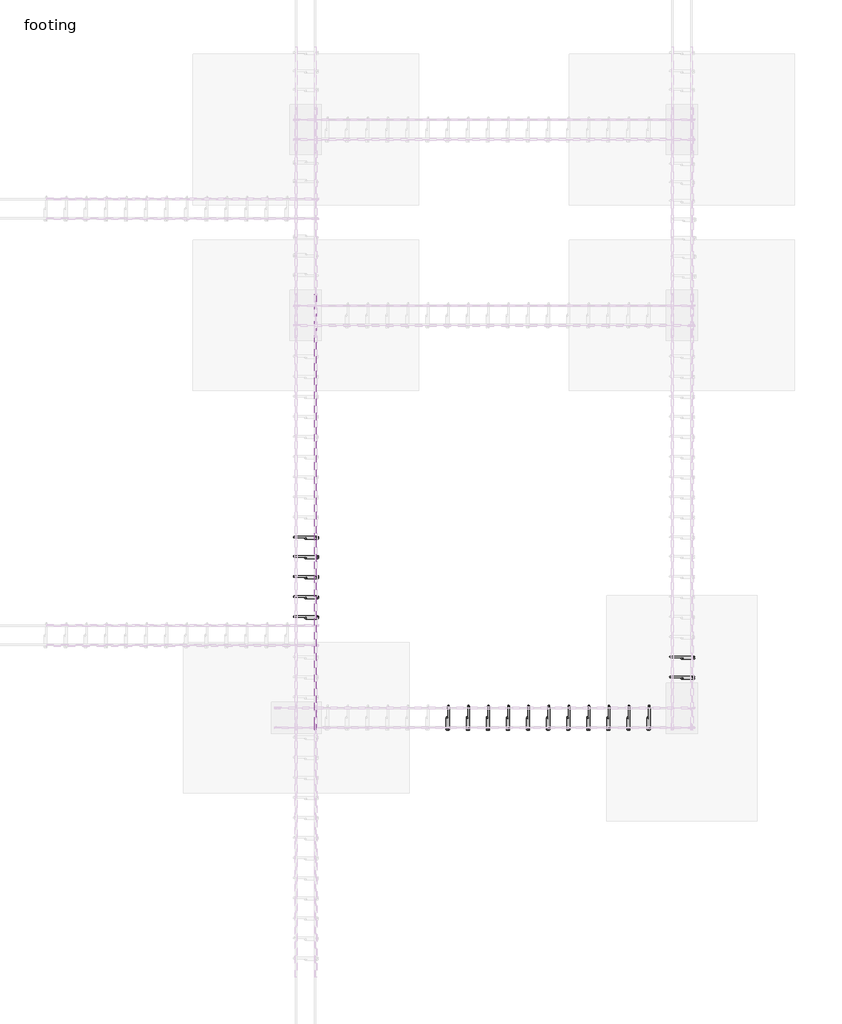
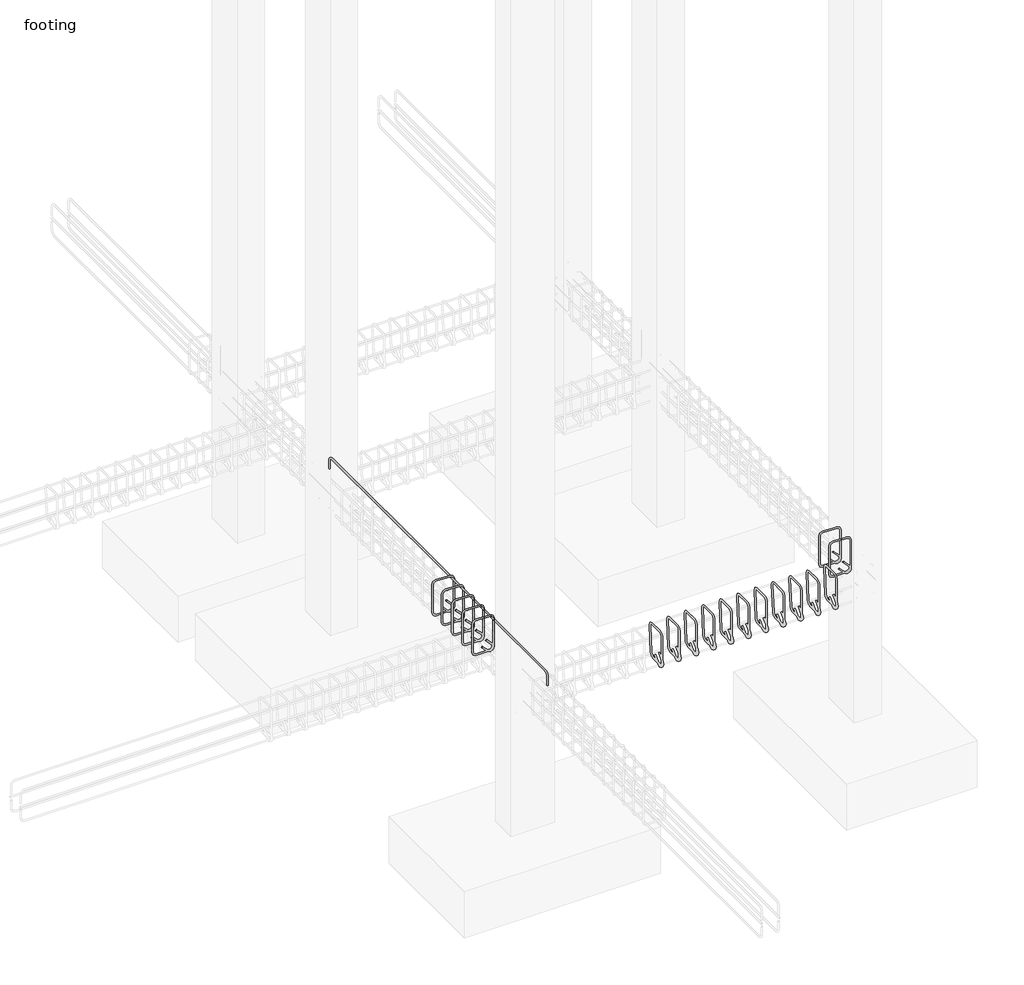
# One storey, part 11 of 21: 19 reinforcing bars.
"""IFC4 building model written with IfcOpenShell, lengths in millimetres."""

from ifc_helpers import new_model, si_unit, point, frame, origin, place, context, project, spatial, polyline, circle_curve, trimmed, segment, composite_curve, element, save
from ifc_brep_helpers import swept_disk

model = new_model("IFC4")

# Units and contexts
model_context = context("Model", 3, world=origin())
ifc_project = project(units=[si_unit("LENGTHUNIT", "METRE", prefix="MILLI")], contexts=[model_context])

# Site, building, storey
site = spatial("IfcSite", under=ifc_project)
building = spatial("IfcBuilding", under=site)
storey = spatial("IfcBuildingStorey", under=building, Name="footing", Elevation=-1524.0)

# Reinforcing bars
placement = place(None, origin())
element("IfcReinforcingBar", 1, at=placement, inside=storey, context=model_context, shape_type="SolidModel", body=[
    swept_disk(composite_curve([segment(polyline([(-6723.5883428, 3451.1387132, -310.8825168), (-6723.5883428, 3396.2737147, -365.7475153)]), True, "CONTINUOUS"), segment(trimmed(circle_curve(frame((-6723.5883428, 3373.8230744, -343.296875), z_axis=(-1.0, 0.0, 0.0), x_axis=(0.0, 22.450640299999577, -22.450640299999975)), 31.75), [point((-6723.5883428, 3396.2737147, -365.7475153))], [point((-6723.5883428, 3342.0730744, -343.296875))], True, "CARTESIAN"), True, "CONTINUOUS"), segment(polyline([(-6723.5883428, 3342.0730744, -343.296875), (-6723.5883428, 3342.0730744, -63.103125)]), True, "CONTINUOUS"), segment(trimmed(circle_curve(frame((-6723.5883428, 3373.8230744, -63.103125), z_axis=(-1.0, 0.0, 0.0), x_axis=(0.0, -31.75, 0.0)), 31.75), [point((-6723.5883428, 3342.0730744, -63.103125))], [point((-6723.5883428, 3373.8230744, -31.353125))], True, "CARTESIAN"), True, "CONTINUOUS"), segment(polyline([(-6723.5883428, 3373.8230744, -31.353125), (-6723.5883428, 3501.6168244, -31.353125)]), True, "CONTINUOUS"), segment(trimmed(circle_curve(frame((-6722.4159328, 3501.6168244, -63.0814712), z_axis=(-0.9993179916193466, 0.0, -0.03692629992126919), x_axis=(-1.1724100000001272, 0.0, 31.728346200000004)), 31.75), [point((-6723.5883428, 3501.6168244, -31.353125))], [point((-6722.4159328, 3533.3668244, -63.0814712))], True, "CARTESIAN"), True, "CONTINUOUS"), segment(polyline([(-6722.4159328, 3533.3668244, -63.0814712), (-6712.0607528, 3533.3668244, -343.3185288)]), True, "CONTINUOUS"), segment(trimmed(circle_curve(frame((-6712.0607528, 3501.6168244, -343.3185288), z_axis=(-0.9993179916193466, 0.0, -0.03692629992126919), x_axis=(0.0, 31.75, 0.0)), 31.75), [point((-6712.0607528, 3533.3668244, -343.3185288))], [point((-6710.8883428, 3501.6168244, -375.046875))], True, "CARTESIAN"), True, "CONTINUOUS"), segment(polyline([(-6710.8883428, 3501.6168244, -375.046875), (-6710.8883428, 3373.8230744, -375.046875)]), True, "CONTINUOUS"), segment(trimmed(circle_curve(frame((-6710.8883428, 3373.8230744, -343.296875), z_axis=(-1.0, 0.0, 0.0), x_axis=(0.0, 0.0, -31.75)), 31.75), [point((-6710.8883428, 3373.8230744, -375.046875))], [point((-6710.8883428, 3351.3724341, -320.8462347))], True, "CARTESIAN"), True, "CONTINUOUS"), segment(polyline([(-6710.8883428, 3351.3724341, -320.8462347), (-6710.8883428, 3406.2374326, -265.9812362)]), True, "CONTINUOUS")], self_intersect=False), 6.35),
])
element("IfcReinforcingBar", 2, at=placement, inside=storey, context=model_context, shape_type="SolidModel", body=[
    swept_disk(composite_curve([segment(polyline([(-6560.8883428, 3451.1387132, -310.8825168), (-6560.8883428, 3396.2737147, -365.7475153)]), True, "CONTINUOUS"), segment(trimmed(circle_curve(frame((-6560.8883428, 3373.8230744, -343.296875), z_axis=(-1.0, 0.0, 0.0), x_axis=(0.0, 22.450640299999577, -22.450640299999975)), 31.75), [point((-6560.8883428, 3396.2737147, -365.7475153))], [point((-6560.8883428, 3342.0730744, -343.296875))], True, "CARTESIAN"), True, "CONTINUOUS"), segment(polyline([(-6560.8883428, 3342.0730744, -343.296875), (-6560.8883428, 3342.0730744, -63.103125)]), True, "CONTINUOUS"), segment(trimmed(circle_curve(frame((-6560.8883428, 3373.8230744, -63.103125), z_axis=(-1.0, 0.0, 0.0), x_axis=(0.0, -31.75, 0.0)), 31.75), [point((-6560.8883428, 3342.0730744, -63.103125))], [point((-6560.8883428, 3373.8230744, -31.353125))], True, "CARTESIAN"), True, "CONTINUOUS"), segment(polyline([(-6560.8883428, 3373.8230744, -31.353125), (-6560.8883428, 3501.6168244, -31.353125)]), True, "CONTINUOUS"), segment(trimmed(circle_curve(frame((-6559.7159328, 3501.6168244, -63.0814712), z_axis=(-0.9993179916193466, 0.0, -0.03692629992126919), x_axis=(-1.1724100000001272, 0.0, 31.728346200000004)), 31.75), [point((-6560.8883428, 3501.6168244, -31.353125))], [point((-6559.7159328, 3533.3668244, -63.0814712))], True, "CARTESIAN"), True, "CONTINUOUS"), segment(polyline([(-6559.7159328, 3533.3668244, -63.0814712), (-6549.3607528, 3533.3668244, -343.3185288)]), True, "CONTINUOUS"), segment(trimmed(circle_curve(frame((-6549.3607528, 3501.6168244, -343.3185288), z_axis=(-0.9993179916193466, 0.0, -0.03692629992126919), x_axis=(0.0, 31.75, 0.0)), 31.75), [point((-6549.3607528, 3533.3668244, -343.3185288))], [point((-6548.1883428, 3501.6168244, -375.046875))], True, "CARTESIAN"), True, "CONTINUOUS"), segment(polyline([(-6548.1883428, 3501.6168244, -375.046875), (-6548.1883428, 3373.8230744, -375.046875)]), True, "CONTINUOUS"), segment(trimmed(circle_curve(frame((-6548.1883428, 3373.8230744, -343.296875), z_axis=(-1.0, 0.0, 0.0), x_axis=(0.0, 0.0, -31.75)), 31.75), [point((-6548.1883428, 3373.8230744, -375.046875))], [point((-6548.1883428, 3351.3724341, -320.8462347))], True, "CARTESIAN"), True, "CONTINUOUS"), segment(polyline([(-6548.1883428, 3351.3724341, -320.8462347), (-6548.1883428, 3406.2374326, -265.9812362)]), True, "CONTINUOUS")], self_intersect=False), 6.35),
])
element("IfcReinforcingBar", 3, at=placement, inside=storey, context=model_context, shape_type="SolidModel", body=[
    swept_disk(composite_curve([segment(polyline([(-6398.1883428, 3451.1387132, -310.8825168), (-6398.1883428, 3396.2737147, -365.7475153)]), True, "CONTINUOUS"), segment(trimmed(circle_curve(frame((-6398.1883428, 3373.8230744, -343.296875), z_axis=(-1.0, 0.0, 0.0), x_axis=(0.0, 22.450640299999577, -22.450640299999975)), 31.75), [point((-6398.1883428, 3396.2737147, -365.7475153))], [point((-6398.1883428, 3342.0730744, -343.296875))], True, "CARTESIAN"), True, "CONTINUOUS"), segment(polyline([(-6398.1883428, 3342.0730744, -343.296875), (-6398.1883428, 3342.0730744, -63.103125)]), True, "CONTINUOUS"), segment(trimmed(circle_curve(frame((-6398.1883428, 3373.8230744, -63.103125), z_axis=(-1.0, 0.0, 0.0), x_axis=(0.0, -31.75, 0.0)), 31.75), [point((-6398.1883428, 3342.0730744, -63.103125))], [point((-6398.1883428, 3373.8230744, -31.353125))], True, "CARTESIAN"), True, "CONTINUOUS"), segment(polyline([(-6398.1883428, 3373.8230744, -31.353125), (-6398.1883428, 3501.6168244, -31.353125)]), True, "CONTINUOUS"), segment(trimmed(circle_curve(frame((-6397.0159328, 3501.6168244, -63.0814712), z_axis=(-0.9993179916193466, 0.0, -0.03692629992126919), x_axis=(-1.1724100000001272, 0.0, 31.728346200000004)), 31.75), [point((-6398.1883428, 3501.6168244, -31.353125))], [point((-6397.0159328, 3533.3668244, -63.0814712))], True, "CARTESIAN"), True, "CONTINUOUS"), segment(polyline([(-6397.0159328, 3533.3668244, -63.0814712), (-6386.6607528, 3533.3668244, -343.3185288)]), True, "CONTINUOUS"), segment(trimmed(circle_curve(frame((-6386.6607528, 3501.6168244, -343.3185288), z_axis=(-0.9993179916193466, 0.0, -0.03692629992126919), x_axis=(0.0, 31.75, 0.0)), 31.75), [point((-6386.6607528, 3533.3668244, -343.3185288))], [point((-6385.4883428, 3501.6168244, -375.046875))], True, "CARTESIAN"), True, "CONTINUOUS"), segment(polyline([(-6385.4883428, 3501.6168244, -375.046875), (-6385.4883428, 3373.8230744, -375.046875)]), True, "CONTINUOUS"), segment(trimmed(circle_curve(frame((-6385.4883428, 3373.8230744, -343.296875), z_axis=(-1.0, 0.0, 0.0), x_axis=(0.0, 0.0, -31.75)), 31.75), [point((-6385.4883428, 3373.8230744, -375.046875))], [point((-6385.4883428, 3351.3724341, -320.8462347))], True, "CARTESIAN"), True, "CONTINUOUS"), segment(polyline([(-6385.4883428, 3351.3724341, -320.8462347), (-6385.4883428, 3406.2374326, -265.9812362)]), True, "CONTINUOUS")], self_intersect=False), 6.35),
])
element("IfcReinforcingBar", 4, at=placement, inside=storey, context=model_context, shape_type="SolidModel", body=[
    swept_disk(composite_curve([segment(polyline([(-6235.4883428, 3451.1387132, -310.8825168), (-6235.4883428, 3396.2737147, -365.7475153)]), True, "CONTINUOUS"), segment(trimmed(circle_curve(frame((-6235.4883428, 3373.8230744, -343.296875), z_axis=(-1.0, 0.0, 0.0), x_axis=(0.0, 22.450640299999577, -22.450640299999975)), 31.75), [point((-6235.4883428, 3396.2737147, -365.7475153))], [point((-6235.4883428, 3342.0730744, -343.296875))], True, "CARTESIAN"), True, "CONTINUOUS"), segment(polyline([(-6235.4883428, 3342.0730744, -343.296875), (-6235.4883428, 3342.0730744, -63.103125)]), True, "CONTINUOUS"), segment(trimmed(circle_curve(frame((-6235.4883428, 3373.8230744, -63.103125), z_axis=(-1.0, 0.0, 0.0), x_axis=(0.0, -31.75, 0.0)), 31.75), [point((-6235.4883428, 3342.0730744, -63.103125))], [point((-6235.4883428, 3373.8230744, -31.353125))], True, "CARTESIAN"), True, "CONTINUOUS"), segment(polyline([(-6235.4883428, 3373.8230744, -31.353125), (-6235.4883428, 3501.6168244, -31.353125)]), True, "CONTINUOUS"), segment(trimmed(circle_curve(frame((-6234.3159328, 3501.6168244, -63.0814712), z_axis=(-0.9993179916193466, 0.0, -0.03692629992126919), x_axis=(-1.1724100000001272, 0.0, 31.728346200000004)), 31.75), [point((-6235.4883428, 3501.6168244, -31.353125))], [point((-6234.3159328, 3533.3668244, -63.0814712))], True, "CARTESIAN"), True, "CONTINUOUS"), segment(polyline([(-6234.3159328, 3533.3668244, -63.0814712), (-6223.9607528, 3533.3668244, -343.3185288)]), True, "CONTINUOUS"), segment(trimmed(circle_curve(frame((-6223.9607528, 3501.6168244, -343.3185288), z_axis=(-0.9993179916193466, 0.0, -0.03692629992126919), x_axis=(0.0, 31.75, 0.0)), 31.75), [point((-6223.9607528, 3533.3668244, -343.3185288))], [point((-6222.7883428, 3501.6168244, -375.046875))], True, "CARTESIAN"), True, "CONTINUOUS"), segment(polyline([(-6222.7883428, 3501.6168244, -375.046875), (-6222.7883428, 3373.8230744, -375.046875)]), True, "CONTINUOUS"), segment(trimmed(circle_curve(frame((-6222.7883428, 3373.8230744, -343.296875), z_axis=(-1.0, 0.0, 0.0), x_axis=(0.0, 0.0, -31.75)), 31.75), [point((-6222.7883428, 3373.8230744, -375.046875))], [point((-6222.7883428, 3351.3724341, -320.8462347))], True, "CARTESIAN"), True, "CONTINUOUS"), segment(polyline([(-6222.7883428, 3351.3724341, -320.8462347), (-6222.7883428, 3406.2374326, -265.9812362)]), True, "CONTINUOUS")], self_intersect=False), 6.35),
])
element("IfcReinforcingBar", 5, at=placement, inside=storey, context=model_context, shape_type="SolidModel", body=[
    swept_disk(composite_curve([segment(polyline([(-6072.7883428, 3451.1387132, -310.8825168), (-6072.7883428, 3396.2737147, -365.7475153)]), True, "CONTINUOUS"), segment(trimmed(circle_curve(frame((-6072.7883428, 3373.8230744, -343.296875), z_axis=(-1.0, 0.0, 0.0), x_axis=(0.0, 22.450640299999577, -22.450640299999975)), 31.75), [point((-6072.7883428, 3396.2737147, -365.7475153))], [point((-6072.7883428, 3342.0730744, -343.296875))], True, "CARTESIAN"), True, "CONTINUOUS"), segment(polyline([(-6072.7883428, 3342.0730744, -343.296875), (-6072.7883428, 3342.0730744, -63.103125)]), True, "CONTINUOUS"), segment(trimmed(circle_curve(frame((-6072.7883428, 3373.8230744, -63.103125), z_axis=(-1.0, 0.0, 0.0), x_axis=(0.0, -31.75, 0.0)), 31.75), [point((-6072.7883428, 3342.0730744, -63.103125))], [point((-6072.7883428, 3373.8230744, -31.353125))], True, "CARTESIAN"), True, "CONTINUOUS"), segment(polyline([(-6072.7883428, 3373.8230744, -31.353125), (-6072.7883428, 3501.6168244, -31.353125)]), True, "CONTINUOUS"), segment(trimmed(circle_curve(frame((-6071.6159328, 3501.6168244, -63.0814712), z_axis=(-0.9993179916193466, 0.0, -0.03692629992126919), x_axis=(-1.1724099999992177, 0.0, 31.728346200000004)), 31.75), [point((-6072.7883428, 3501.6168244, -31.353125))], [point((-6071.6159328, 3533.3668244, -63.0814712))], True, "CARTESIAN"), True, "CONTINUOUS"), segment(polyline([(-6071.6159328, 3533.3668244, -63.0814712), (-6061.2607528, 3533.3668244, -343.3185288)]), True, "CONTINUOUS"), segment(trimmed(circle_curve(frame((-6061.2607528, 3501.6168244, -343.3185288), z_axis=(-0.9993179916193466, 0.0, -0.03692629992126919), x_axis=(0.0, 31.75, 0.0)), 31.75), [point((-6061.2607528, 3533.3668244, -343.3185288))], [point((-6060.0883428, 3501.6168244, -375.046875))], True, "CARTESIAN"), True, "CONTINUOUS"), segment(polyline([(-6060.0883428, 3501.6168244, -375.046875), (-6060.0883428, 3373.8230744, -375.046875)]), True, "CONTINUOUS"), segment(trimmed(circle_curve(frame((-6060.0883428, 3373.8230744, -343.296875), z_axis=(-1.0, 0.0, 0.0), x_axis=(0.0, 0.0, -31.75)), 31.75), [point((-6060.0883428, 3373.8230744, -375.046875))], [point((-6060.0883428, 3351.3724341, -320.8462347))], True, "CARTESIAN"), True, "CONTINUOUS"), segment(polyline([(-6060.0883428, 3351.3724341, -320.8462347), (-6060.0883428, 3406.2374326, -265.9812362)]), True, "CONTINUOUS")], self_intersect=False), 6.35),
])
element("IfcReinforcingBar", 6, at=placement, inside=storey, context=model_context, shape_type="SolidModel", body=[
    swept_disk(composite_curve([segment(polyline([(-5910.0883428, 3451.1387132, -310.8825168), (-5910.0883428, 3396.2737147, -365.7475153)]), True, "CONTINUOUS"), segment(trimmed(circle_curve(frame((-5910.0883428, 3373.8230744, -343.296875), z_axis=(-1.0, 0.0, 0.0), x_axis=(0.0, 22.450640299999577, -22.450640299999975)), 31.75), [point((-5910.0883428, 3396.2737147, -365.7475153))], [point((-5910.0883428, 3342.0730744, -343.296875))], True, "CARTESIAN"), True, "CONTINUOUS"), segment(polyline([(-5910.0883428, 3342.0730744, -343.296875), (-5910.0883428, 3342.0730744, -63.103125)]), True, "CONTINUOUS"), segment(trimmed(circle_curve(frame((-5910.0883428, 3373.8230744, -63.103125), z_axis=(-1.0, 0.0, 0.0), x_axis=(0.0, -31.75, 0.0)), 31.75), [point((-5910.0883428, 3342.0730744, -63.103125))], [point((-5910.0883428, 3373.8230744, -31.353125))], True, "CARTESIAN"), True, "CONTINUOUS"), segment(polyline([(-5910.0883428, 3373.8230744, -31.353125), (-5910.0883428, 3501.6168244, -31.353125)]), True, "CONTINUOUS"), segment(trimmed(circle_curve(frame((-5908.9159328, 3501.6168244, -63.0814712), z_axis=(-0.9993179916193466, 0.0, -0.03692629992126919), x_axis=(-1.1724100000001272, 0.0, 31.728346200000004)), 31.75), [point((-5910.0883428, 3501.6168244, -31.353125))], [point((-5908.9159328, 3533.3668244, -63.0814712))], True, "CARTESIAN"), True, "CONTINUOUS"), segment(polyline([(-5908.9159328, 3533.3668244, -63.0814712), (-5898.5607528, 3533.3668244, -343.3185288)]), True, "CONTINUOUS"), segment(trimmed(circle_curve(frame((-5898.5607528, 3501.6168244, -343.3185288), z_axis=(-0.9993179916193466, 0.0, -0.03692629992126919), x_axis=(0.0, 31.75, 0.0)), 31.75), [point((-5898.5607528, 3533.3668244, -343.3185288))], [point((-5897.3883428, 3501.6168244, -375.046875))], True, "CARTESIAN"), True, "CONTINUOUS"), segment(polyline([(-5897.3883428, 3501.6168244, -375.046875), (-5897.3883428, 3373.8230744, -375.046875)]), True, "CONTINUOUS"), segment(trimmed(circle_curve(frame((-5897.3883428, 3373.8230744, -343.296875), z_axis=(-1.0, 0.0, 0.0), x_axis=(0.0, 0.0, -31.75)), 31.75), [point((-5897.3883428, 3373.8230744, -375.046875))], [point((-5897.3883428, 3351.3724341, -320.8462347))], True, "CARTESIAN"), True, "CONTINUOUS"), segment(polyline([(-5897.3883428, 3351.3724341, -320.8462347), (-5897.3883428, 3406.2374326, -265.9812362)]), True, "CONTINUOUS")], self_intersect=False), 6.35),
])
element("IfcReinforcingBar", 7, at=placement, inside=storey, context=model_context, shape_type="SolidModel", body=[
    swept_disk(composite_curve([segment(polyline([(-5747.3883428, 3451.1387132, -310.8825168), (-5747.3883428, 3396.2737147, -365.7475153)]), True, "CONTINUOUS"), segment(trimmed(circle_curve(frame((-5747.3883428, 3373.8230744, -343.296875), z_axis=(-1.0, 0.0, 0.0), x_axis=(0.0, 22.450640299999577, -22.450640299999975)), 31.75), [point((-5747.3883428, 3396.2737147, -365.7475153))], [point((-5747.3883428, 3342.0730744, -343.296875))], True, "CARTESIAN"), True, "CONTINUOUS"), segment(polyline([(-5747.3883428, 3342.0730744, -343.296875), (-5747.3883428, 3342.0730744, -63.103125)]), True, "CONTINUOUS"), segment(trimmed(circle_curve(frame((-5747.3883428, 3373.8230744, -63.103125), z_axis=(-1.0, 0.0, 0.0), x_axis=(0.0, -31.75, 0.0)), 31.75), [point((-5747.3883428, 3342.0730744, -63.103125))], [point((-5747.3883428, 3373.8230744, -31.353125))], True, "CARTESIAN"), True, "CONTINUOUS"), segment(polyline([(-5747.3883428, 3373.8230744, -31.353125), (-5747.3883428, 3501.6168244, -31.353125)]), True, "CONTINUOUS"), segment(trimmed(circle_curve(frame((-5746.2159328, 3501.6168244, -63.0814712), z_axis=(-0.9993179916193466, 0.0, -0.03692629992126919), x_axis=(-1.1724100000001272, 0.0, 31.728346200000004)), 31.75), [point((-5747.3883428, 3501.6168244, -31.353125))], [point((-5746.2159328, 3533.3668244, -63.0814712))], True, "CARTESIAN"), True, "CONTINUOUS"), segment(polyline([(-5746.2159328, 3533.3668244, -63.0814712), (-5735.8607528, 3533.3668244, -343.3185288)]), True, "CONTINUOUS"), segment(trimmed(circle_curve(frame((-5735.8607528, 3501.6168244, -343.3185288), z_axis=(-0.9993179916193466, 0.0, -0.03692629992126919), x_axis=(0.0, 31.75, 0.0)), 31.75), [point((-5735.8607528, 3533.3668244, -343.3185288))], [point((-5734.6883428, 3501.6168244, -375.046875))], True, "CARTESIAN"), True, "CONTINUOUS"), segment(polyline([(-5734.6883428, 3501.6168244, -375.046875), (-5734.6883428, 3373.8230744, -375.046875)]), True, "CONTINUOUS"), segment(trimmed(circle_curve(frame((-5734.6883428, 3373.8230744, -343.296875), z_axis=(-1.0, 0.0, 0.0), x_axis=(0.0, 0.0, -31.75)), 31.75), [point((-5734.6883428, 3373.8230744, -375.046875))], [point((-5734.6883428, 3351.3724341, -320.8462347))], True, "CARTESIAN"), True, "CONTINUOUS"), segment(polyline([(-5734.6883428, 3351.3724341, -320.8462347), (-5734.6883428, 3406.2374326, -265.9812362)]), True, "CONTINUOUS")], self_intersect=False), 6.35),
])
element("IfcReinforcingBar", 8, at=placement, inside=storey, context=model_context, shape_type="SolidModel", body=[
    swept_disk(composite_curve([segment(polyline([(-5584.6883428, 3451.1387132, -310.8825168), (-5584.6883428, 3396.2737147, -365.7475153)]), True, "CONTINUOUS"), segment(trimmed(circle_curve(frame((-5584.6883428, 3373.8230744, -343.296875), z_axis=(-1.0, 0.0, 0.0), x_axis=(0.0, 22.450640299999577, -22.450640299999975)), 31.75), [point((-5584.6883428, 3396.2737147, -365.7475153))], [point((-5584.6883428, 3342.0730744, -343.296875))], True, "CARTESIAN"), True, "CONTINUOUS"), segment(polyline([(-5584.6883428, 3342.0730744, -343.296875), (-5584.6883428, 3342.0730744, -63.103125)]), True, "CONTINUOUS"), segment(trimmed(circle_curve(frame((-5584.6883428, 3373.8230744, -63.103125), z_axis=(-1.0, 0.0, 0.0), x_axis=(0.0, -31.75, 0.0)), 31.75), [point((-5584.6883428, 3342.0730744, -63.103125))], [point((-5584.6883428, 3373.8230744, -31.353125))], True, "CARTESIAN"), True, "CONTINUOUS"), segment(polyline([(-5584.6883428, 3373.8230744, -31.353125), (-5584.6883428, 3501.6168244, -31.353125)]), True, "CONTINUOUS"), segment(trimmed(circle_curve(frame((-5583.5159328, 3501.6168244, -63.0814712), z_axis=(-0.9993179916193466, 0.0, -0.03692629992126919), x_axis=(-1.1724100000001272, 0.0, 31.728346200000004)), 31.75), [point((-5584.6883428, 3501.6168244, -31.353125))], [point((-5583.5159328, 3533.3668244, -63.0814712))], True, "CARTESIAN"), True, "CONTINUOUS"), segment(polyline([(-5583.5159328, 3533.3668244, -63.0814712), (-5573.1607528, 3533.3668244, -343.3185288)]), True, "CONTINUOUS"), segment(trimmed(circle_curve(frame((-5573.1607528, 3501.6168244, -343.3185288), z_axis=(-0.9993179916193466, 0.0, -0.03692629992126919), x_axis=(0.0, 31.75, 0.0)), 31.75), [point((-5573.1607528, 3533.3668244, -343.3185288))], [point((-5571.9883428, 3501.6168244, -375.046875))], True, "CARTESIAN"), True, "CONTINUOUS"), segment(polyline([(-5571.9883428, 3501.6168244, -375.046875), (-5571.9883428, 3373.8230744, -375.046875)]), True, "CONTINUOUS"), segment(trimmed(circle_curve(frame((-5571.9883428, 3373.8230744, -343.296875), z_axis=(-1.0, 0.0, 0.0), x_axis=(0.0, 0.0, -31.75)), 31.75), [point((-5571.9883428, 3373.8230744, -375.046875))], [point((-5571.9883428, 3351.3724341, -320.8462347))], True, "CARTESIAN"), True, "CONTINUOUS"), segment(polyline([(-5571.9883428, 3351.3724341, -320.8462347), (-5571.9883428, 3406.2374326, -265.9812362)]), True, "CONTINUOUS")], self_intersect=False), 6.35),
])
element("IfcReinforcingBar", 9, at=placement, inside=storey, context=model_context, shape_type="SolidModel", body=[
    swept_disk(composite_curve([segment(polyline([(-5421.9883428, 3451.1387132, -310.8825168), (-5421.9883428, 3396.2737147, -365.7475153)]), True, "CONTINUOUS"), segment(trimmed(circle_curve(frame((-5421.9883428, 3373.8230744, -343.296875), z_axis=(-1.0, 0.0, 0.0), x_axis=(0.0, 22.450640299999577, -22.450640299999975)), 31.75), [point((-5421.9883428, 3396.2737147, -365.7475153))], [point((-5421.9883428, 3342.0730744, -343.296875))], True, "CARTESIAN"), True, "CONTINUOUS"), segment(polyline([(-5421.9883428, 3342.0730744, -343.296875), (-5421.9883428, 3342.0730744, -63.103125)]), True, "CONTINUOUS"), segment(trimmed(circle_curve(frame((-5421.9883428, 3373.8230744, -63.103125), z_axis=(-1.0, 0.0, 0.0), x_axis=(0.0, -31.75, 0.0)), 31.75), [point((-5421.9883428, 3342.0730744, -63.103125))], [point((-5421.9883428, 3373.8230744, -31.353125))], True, "CARTESIAN"), True, "CONTINUOUS"), segment(polyline([(-5421.9883428, 3373.8230744, -31.353125), (-5421.9883428, 3501.6168244, -31.353125)]), True, "CONTINUOUS"), segment(trimmed(circle_curve(frame((-5420.8159328, 3501.6168244, -63.0814712), z_axis=(-0.9993179916193466, 0.0, -0.03692629992126919), x_axis=(-1.1724100000001272, 0.0, 31.728346200000004)), 31.75), [point((-5421.9883428, 3501.6168244, -31.353125))], [point((-5420.8159328, 3533.3668244, -63.0814712))], True, "CARTESIAN"), True, "CONTINUOUS"), segment(polyline([(-5420.8159328, 3533.3668244, -63.0814712), (-5410.4607528, 3533.3668244, -343.3185288)]), True, "CONTINUOUS"), segment(trimmed(circle_curve(frame((-5410.4607528, 3501.6168244, -343.3185288), z_axis=(-0.9993179916193466, 0.0, -0.03692629992126919), x_axis=(0.0, 31.75, 0.0)), 31.75), [point((-5410.4607528, 3533.3668244, -343.3185288))], [point((-5409.2883428, 3501.6168244, -375.046875))], True, "CARTESIAN"), True, "CONTINUOUS"), segment(polyline([(-5409.2883428, 3501.6168244, -375.046875), (-5409.2883428, 3373.8230744, -375.046875)]), True, "CONTINUOUS"), segment(trimmed(circle_curve(frame((-5409.2883428, 3373.8230744, -343.296875), z_axis=(-1.0, 0.0, 0.0), x_axis=(0.0, 0.0, -31.75)), 31.75), [point((-5409.2883428, 3373.8230744, -375.046875))], [point((-5409.2883428, 3351.3724341, -320.8462347))], True, "CARTESIAN"), True, "CONTINUOUS"), segment(polyline([(-5409.2883428, 3351.3724341, -320.8462347), (-5409.2883428, 3406.2374326, -265.9812362)]), True, "CONTINUOUS")], self_intersect=False), 6.35),
])
element("IfcReinforcingBar", 10, at=placement, inside=storey, context=model_context, shape_type="SolidModel", body=[
    swept_disk(composite_curve([segment(polyline([(-5259.2883428, 3451.1387132, -310.8825168), (-5259.2883428, 3396.2737147, -365.7475153)]), True, "CONTINUOUS"), segment(trimmed(circle_curve(frame((-5259.2883428, 3373.8230744, -343.296875), z_axis=(-1.0, 0.0, 0.0), x_axis=(0.0, 22.450640299999577, -22.450640299999975)), 31.75), [point((-5259.2883428, 3396.2737147, -365.7475153))], [point((-5259.2883428, 3342.0730744, -343.296875))], True, "CARTESIAN"), True, "CONTINUOUS"), segment(polyline([(-5259.2883428, 3342.0730744, -343.296875), (-5259.2883428, 3342.0730744, -63.103125)]), True, "CONTINUOUS"), segment(trimmed(circle_curve(frame((-5259.2883428, 3373.8230744, -63.103125), z_axis=(-1.0, 0.0, 0.0), x_axis=(0.0, -31.75, 0.0)), 31.75), [point((-5259.2883428, 3342.0730744, -63.103125))], [point((-5259.2883428, 3373.8230744, -31.353125))], True, "CARTESIAN"), True, "CONTINUOUS"), segment(polyline([(-5259.2883428, 3373.8230744, -31.353125), (-5259.2883428, 3501.6168244, -31.353125)]), True, "CONTINUOUS"), segment(trimmed(circle_curve(frame((-5258.1159328, 3501.6168244, -63.0814712), z_axis=(-0.9993179916193466, 0.0, -0.03692629992126919), x_axis=(-1.1724099999992177, 0.0, 31.728346200000004)), 31.75), [point((-5259.2883428, 3501.6168244, -31.353125))], [point((-5258.1159328, 3533.3668244, -63.0814712))], True, "CARTESIAN"), True, "CONTINUOUS"), segment(polyline([(-5258.1159328, 3533.3668244, -63.0814712), (-5247.7607528, 3533.3668244, -343.3185288)]), True, "CONTINUOUS"), segment(trimmed(circle_curve(frame((-5247.7607528, 3501.6168244, -343.3185288), z_axis=(-0.9993179916193466, 0.0, -0.03692629992126919), x_axis=(0.0, 31.75, 0.0)), 31.75), [point((-5247.7607528, 3533.3668244, -343.3185288))], [point((-5246.5883428, 3501.6168244, -375.046875))], True, "CARTESIAN"), True, "CONTINUOUS"), segment(polyline([(-5246.5883428, 3501.6168244, -375.046875), (-5246.5883428, 3373.8230744, -375.046875)]), True, "CONTINUOUS"), segment(trimmed(circle_curve(frame((-5246.5883428, 3373.8230744, -343.296875), z_axis=(-1.0, 0.0, 0.0), x_axis=(0.0, 0.0, -31.75)), 31.75), [point((-5246.5883428, 3373.8230744, -375.046875))], [point((-5246.5883428, 3351.3724341, -320.8462347))], True, "CARTESIAN"), True, "CONTINUOUS"), segment(polyline([(-5246.5883428, 3351.3724341, -320.8462347), (-5246.5883428, 3406.2374326, -265.9812362)]), True, "CONTINUOUS")], self_intersect=False), 6.35),
])
element("IfcReinforcingBar", 11, at=placement, inside=storey, context=model_context, shape_type="SolidModel", body=[
    swept_disk(composite_curve([segment(polyline([(-5096.5883428, 3451.1387132, -310.8825168), (-5096.5883428, 3396.2737147, -365.7475153)]), True, "CONTINUOUS"), segment(trimmed(circle_curve(frame((-5096.5883428, 3373.8230744, -343.296875), z_axis=(-1.0, 0.0, 0.0), x_axis=(0.0, 22.450640299999577, -22.450640299999975)), 31.75), [point((-5096.5883428, 3396.2737147, -365.7475153))], [point((-5096.5883428, 3342.0730744, -343.296875))], True, "CARTESIAN"), True, "CONTINUOUS"), segment(polyline([(-5096.5883428, 3342.0730744, -343.296875), (-5096.5883428, 3342.0730744, -63.103125)]), True, "CONTINUOUS"), segment(trimmed(circle_curve(frame((-5096.5883428, 3373.8230744, -63.103125), z_axis=(-1.0, 0.0, 0.0), x_axis=(0.0, -31.75, 0.0)), 31.75), [point((-5096.5883428, 3342.0730744, -63.103125))], [point((-5096.5883428, 3373.8230744, -31.353125))], True, "CARTESIAN"), True, "CONTINUOUS"), segment(polyline([(-5096.5883428, 3373.8230744, -31.353125), (-5096.5883428, 3501.6168244, -31.353125)]), True, "CONTINUOUS"), segment(trimmed(circle_curve(frame((-5095.4159328, 3501.6168244, -63.0814712), z_axis=(-0.9993179916193466, 0.0, -0.03692629992126919), x_axis=(-1.1724100000001272, 0.0, 31.728346200000004)), 31.75), [point((-5096.5883428, 3501.6168244, -31.353125))], [point((-5095.4159328, 3533.3668244, -63.0814712))], True, "CARTESIAN"), True, "CONTINUOUS"), segment(polyline([(-5095.4159328, 3533.3668244, -63.0814712), (-5085.0607528, 3533.3668244, -343.3185288)]), True, "CONTINUOUS"), segment(trimmed(circle_curve(frame((-5085.0607528, 3501.6168244, -343.3185288), z_axis=(-0.9993179916193466, 0.0, -0.03692629992126919), x_axis=(0.0, 31.75, 0.0)), 31.75), [point((-5085.0607528, 3533.3668244, -343.3185288))], [point((-5083.8883428, 3501.6168244, -375.046875))], True, "CARTESIAN"), True, "CONTINUOUS"), segment(polyline([(-5083.8883428, 3501.6168244, -375.046875), (-5083.8883428, 3373.8230744, -375.046875)]), True, "CONTINUOUS"), segment(trimmed(circle_curve(frame((-5083.8883428, 3373.8230744, -343.296875), z_axis=(-1.0, 0.0, 0.0), x_axis=(0.0, 0.0, -31.75)), 31.75), [point((-5083.8883428, 3373.8230744, -375.046875))], [point((-5083.8883428, 3351.3724341, -320.8462347))], True, "CARTESIAN"), True, "CONTINUOUS"), segment(polyline([(-5083.8883428, 3351.3724341, -320.8462347), (-5083.8883428, 3406.2374326, -265.9812362)]), True, "CONTINUOUS")], self_intersect=False), 6.35),
])
element("IfcReinforcingBar", 12, at=placement, inside=storey, context=model_context, shape_type="SolidModel", body=[
    swept_disk(composite_curve([segment(polyline([(-7788.8317831, 3342.0730744, -170.2827408), (-7788.8317831, 3342.0730744, -94.0827408)]), True, "CONTINUOUS"), segment(trimmed(circle_curve(frame((-7788.8317831, 3386.5230744, -94.0827408), z_axis=(-1.0, 0.0, 0.0), x_axis=(0.0, -44.44999999999982, 0.0)), 44.45), [point((-7788.8317831, 3342.0730744, -94.0827408))], [point((-7788.8317831, 3386.5230744, -49.6327408))], True, "CARTESIAN"), True, "CONTINUOUS"), segment(polyline([(-7788.8317831, 3386.5230744, -49.6327408), (-7788.8317831, 6822.6668244, -49.6327408)]), True, "CONTINUOUS"), segment(trimmed(circle_curve(frame((-7788.8317831, 6822.6668244, -94.0827408), z_axis=(-1.0, 0.0, 0.0), x_axis=(0.0, 0.0, 44.449999999999996)), 44.45), [point((-7788.8317831, 6822.6668244, -49.6327408))], [point((-7788.8317831, 6867.1168244, -94.0827408))], True, "CARTESIAN"), True, "CONTINUOUS"), segment(polyline([(-7788.8317831, 6867.1168244, -94.0827408), (-7788.8317831, 6867.1168244, -170.2827408)]), True, "CONTINUOUS")], self_intersect=False), 6.35),
])
element("IfcReinforcingBar", 13, at=placement, inside=storey, context=model_context, shape_type="SolidModel", body=[
    swept_disk(composite_curve([segment(polyline([(-7834.7165254, 4257.0956073, -265.9812362), (-7779.851527, 4257.0956073, -320.8462347)]), True, "CONTINUOUS"), segment(trimmed(circle_curve(frame((-7802.3021673, 4257.0956073, -343.296875), z_axis=(0.0, 1.0, 0.0), x_axis=(22.450640300000487, 0.0, 22.450640299999975)), 31.75), [point((-7779.851527, 4257.0956073, -320.8462347))], [point((-7802.3021673, 4257.0956073, -375.046875))], True, "CARTESIAN"), True, "CONTINUOUS"), segment(polyline([(-7802.3021673, 4257.0956073, -375.046875), (-7930.0959173, 4257.0956073, -375.046875)]), True, "CONTINUOUS"), segment(trimmed(circle_curve(frame((-7930.0959173, 4257.0956073, -343.296875), z_axis=(0.0, 1.0, 0.0), x_axis=(0.0, 0.0, -31.75)), 31.75), [point((-7930.0959173, 4257.0956073, -375.046875))], [point((-7961.8459173, 4257.0956073, -343.296875))], True, "CARTESIAN"), True, "CONTINUOUS"), segment(polyline([(-7961.8459173, 4257.0956073, -343.296875), (-7961.8459173, 4257.0956073, -63.103125)]), True, "CONTINUOUS"), segment(trimmed(circle_curve(frame((-7930.165658, 4254.9923536, -63.103125), z_axis=(0.0662442117686417, 0.9978034397651431, 0.0), x_axis=(-31.680259300000216, 2.1032537000000957, 0.0)), 31.75), [point((-7961.8459173, 4257.0956073, -63.103125))], [point((-7930.165658, 4254.9923536, -31.353125))], True, "CARTESIAN"), True, "CONTINUOUS"), segment(polyline([(-7930.165658, 4254.9923536, -31.353125), (-7802.2324265, 4246.498861, -31.353125)]), True, "CONTINUOUS"), segment(trimmed(circle_curve(frame((-7802.2324265, 4246.498861, -63.103125), z_axis=(0.06624421176864169, 0.997803439765143, 0.0), x_axis=(0.0, 0.0, 31.75)), 31.75), [point((-7802.2324265, 4246.498861, -31.353125))], [point((-7770.5521673, 4244.3956073, -63.103125))], True, "CARTESIAN"), True, "CONTINUOUS"), segment(polyline([(-7770.5521673, 4244.3956073, -63.103125), (-7770.5521673, 4244.3956073, -343.296875)]), True, "CONTINUOUS"), segment(trimmed(circle_curve(frame((-7802.3021673, 4244.3956073, -343.296875), z_axis=(0.0, 1.0, 0.0), x_axis=(31.75, 0.0, 0.0)), 31.75), [point((-7770.5521673, 4244.3956073, -343.296875))], [point((-7824.7528076, 4244.3956073, -365.7475153))], True, "CARTESIAN"), True, "CONTINUOUS"), segment(polyline([(-7824.7528076, 4244.3956073, -365.7475153), (-7879.617806, 4244.3956073, -310.8825168)]), True, "CONTINUOUS")], self_intersect=False), 6.35),
])
element("IfcReinforcingBar", 14, at=placement, inside=storey, context=model_context, shape_type="SolidModel", body=[
    swept_disk(composite_curve([segment(polyline([(-7834.7165254, 4419.7956073, -265.9812362), (-7779.851527, 4419.7956073, -320.8462347)]), True, "CONTINUOUS"), segment(trimmed(circle_curve(frame((-7802.3021673, 4419.7956073, -343.296875), z_axis=(0.0, 1.0, 0.0), x_axis=(22.450640300000487, 0.0, 22.450640299999975)), 31.75), [point((-7779.851527, 4419.7956073, -320.8462347))], [point((-7802.3021673, 4419.7956073, -375.046875))], True, "CARTESIAN"), True, "CONTINUOUS"), segment(polyline([(-7802.3021673, 4419.7956073, -375.046875), (-7930.0959173, 4419.7956073, -375.046875)]), True, "CONTINUOUS"), segment(trimmed(circle_curve(frame((-7930.0959173, 4419.7956073, -343.296875), z_axis=(0.0, 1.0, 0.0), x_axis=(0.0, 0.0, -31.75)), 31.75), [point((-7930.0959173, 4419.7956073, -375.046875))], [point((-7961.8459173, 4419.7956073, -343.296875))], True, "CARTESIAN"), True, "CONTINUOUS"), segment(polyline([(-7961.8459173, 4419.7956073, -343.296875), (-7961.8459173, 4419.7956073, -63.103125)]), True, "CONTINUOUS"), segment(trimmed(circle_curve(frame((-7930.165658, 4417.6923536, -63.103125), z_axis=(0.0662442117686417, 0.9978034397651431, 0.0), x_axis=(-31.680259300000216, 2.103253699999186, 0.0)), 31.75), [point((-7961.8459173, 4419.7956073, -63.103125))], [point((-7930.165658, 4417.6923536, -31.353125))], True, "CARTESIAN"), True, "CONTINUOUS"), segment(polyline([(-7930.165658, 4417.6923536, -31.353125), (-7802.2324265, 4409.198861, -31.353125)]), True, "CONTINUOUS"), segment(trimmed(circle_curve(frame((-7802.2324265, 4409.198861, -63.103125), z_axis=(0.06624421176864169, 0.997803439765143, 0.0), x_axis=(0.0, 0.0, 31.75)), 31.75), [point((-7802.2324265, 4409.198861, -31.353125))], [point((-7770.5521673, 4407.0956073, -63.103125))], True, "CARTESIAN"), True, "CONTINUOUS"), segment(polyline([(-7770.5521673, 4407.0956073, -63.103125), (-7770.5521673, 4407.0956073, -343.296875)]), True, "CONTINUOUS"), segment(trimmed(circle_curve(frame((-7802.3021673, 4407.0956073, -343.296875), z_axis=(0.0, 1.0, 0.0), x_axis=(31.75, 0.0, 0.0)), 31.75), [point((-7770.5521673, 4407.0956073, -343.296875))], [point((-7824.7528076, 4407.0956073, -365.7475153))], True, "CARTESIAN"), True, "CONTINUOUS"), segment(polyline([(-7824.7528076, 4407.0956073, -365.7475153), (-7879.617806, 4407.0956073, -310.8825168)]), True, "CONTINUOUS")], self_intersect=False), 6.35),
])
element("IfcReinforcingBar", 15, at=placement, inside=storey, context=model_context, shape_type="SolidModel", body=[
    swept_disk(composite_curve([segment(polyline([(-7834.7165254, 4582.4956073, -265.9812362), (-7779.851527, 4582.4956073, -320.8462347)]), True, "CONTINUOUS"), segment(trimmed(circle_curve(frame((-7802.3021673, 4582.4956073, -343.296875), z_axis=(0.0, 1.0, 0.0), x_axis=(22.450640300000487, 0.0, 22.450640299999975)), 31.75), [point((-7779.851527, 4582.4956073, -320.8462347))], [point((-7802.3021673, 4582.4956073, -375.046875))], True, "CARTESIAN"), True, "CONTINUOUS"), segment(polyline([(-7802.3021673, 4582.4956073, -375.046875), (-7930.0959173, 4582.4956073, -375.046875)]), True, "CONTINUOUS"), segment(trimmed(circle_curve(frame((-7930.0959173, 4582.4956073, -343.296875), z_axis=(0.0, 1.0, 0.0), x_axis=(0.0, 0.0, -31.75)), 31.75), [point((-7930.0959173, 4582.4956073, -375.046875))], [point((-7961.8459173, 4582.4956073, -343.296875))], True, "CARTESIAN"), True, "CONTINUOUS"), segment(polyline([(-7961.8459173, 4582.4956073, -343.296875), (-7961.8459173, 4582.4956073, -63.103125)]), True, "CONTINUOUS"), segment(trimmed(circle_curve(frame((-7930.165658, 4580.3923536, -63.103125), z_axis=(0.0662442117686417, 0.9978034397651431, 0.0), x_axis=(-31.680259300000216, 2.1032537000000957, 0.0)), 31.75), [point((-7961.8459173, 4582.4956073, -63.103125))], [point((-7930.165658, 4580.3923536, -31.353125))], True, "CARTESIAN"), True, "CONTINUOUS"), segment(polyline([(-7930.165658, 4580.3923536, -31.353125), (-7802.2324265, 4571.898861, -31.353125)]), True, "CONTINUOUS"), segment(trimmed(circle_curve(frame((-7802.2324265, 4571.898861, -63.103125), z_axis=(0.06624421176864169, 0.997803439765143, 0.0), x_axis=(0.0, 0.0, 31.75)), 31.75), [point((-7802.2324265, 4571.898861, -31.353125))], [point((-7770.5521673, 4569.7956073, -63.103125))], True, "CARTESIAN"), True, "CONTINUOUS"), segment(polyline([(-7770.5521673, 4569.7956073, -63.103125), (-7770.5521673, 4569.7956073, -343.296875)]), True, "CONTINUOUS"), segment(trimmed(circle_curve(frame((-7802.3021673, 4569.7956073, -343.296875), z_axis=(0.0, 1.0, 0.0), x_axis=(31.75, 0.0, 0.0)), 31.75), [point((-7770.5521673, 4569.7956073, -343.296875))], [point((-7824.7528076, 4569.7956073, -365.7475153))], True, "CARTESIAN"), True, "CONTINUOUS"), segment(polyline([(-7824.7528076, 4569.7956073, -365.7475153), (-7879.617806, 4569.7956073, -310.8825168)]), True, "CONTINUOUS")], self_intersect=False), 6.35),
])
element("IfcReinforcingBar", 16, at=placement, inside=storey, context=model_context, shape_type="SolidModel", body=[
    swept_disk(composite_curve([segment(polyline([(-7834.7165254, 4745.1956073, -265.9812362), (-7779.851527, 4745.1956073, -320.8462347)]), True, "CONTINUOUS"), segment(trimmed(circle_curve(frame((-7802.3021673, 4745.1956073, -343.296875), z_axis=(0.0, 1.0, 0.0), x_axis=(22.450640300000487, 0.0, 22.450640299999975)), 31.75), [point((-7779.851527, 4745.1956073, -320.8462347))], [point((-7802.3021673, 4745.1956073, -375.046875))], True, "CARTESIAN"), True, "CONTINUOUS"), segment(polyline([(-7802.3021673, 4745.1956073, -375.046875), (-7930.0959173, 4745.1956073, -375.046875)]), True, "CONTINUOUS"), segment(trimmed(circle_curve(frame((-7930.0959173, 4745.1956073, -343.296875), z_axis=(0.0, 1.0, 0.0), x_axis=(0.0, 0.0, -31.75)), 31.75), [point((-7930.0959173, 4745.1956073, -375.046875))], [point((-7961.8459173, 4745.1956073, -343.296875))], True, "CARTESIAN"), True, "CONTINUOUS"), segment(polyline([(-7961.8459173, 4745.1956073, -343.296875), (-7961.8459173, 4745.1956073, -63.103125)]), True, "CONTINUOUS"), segment(trimmed(circle_curve(frame((-7930.165658, 4743.0923536, -63.103125), z_axis=(0.0662442117686417, 0.9978034397651431, 0.0), x_axis=(-31.680259300000216, 2.1032537000000957, 0.0)), 31.75), [point((-7961.8459173, 4745.1956073, -63.103125))], [point((-7930.165658, 4743.0923536, -31.353125))], True, "CARTESIAN"), True, "CONTINUOUS"), segment(polyline([(-7930.165658, 4743.0923536, -31.353125), (-7802.2324265, 4734.598861, -31.353125)]), True, "CONTINUOUS"), segment(trimmed(circle_curve(frame((-7802.2324265, 4734.598861, -63.103125), z_axis=(0.06624421176864169, 0.997803439765143, 0.0), x_axis=(0.0, 0.0, 31.75)), 31.75), [point((-7802.2324265, 4734.598861, -31.353125))], [point((-7770.5521673, 4732.4956073, -63.103125))], True, "CARTESIAN"), True, "CONTINUOUS"), segment(polyline([(-7770.5521673, 4732.4956073, -63.103125), (-7770.5521673, 4732.4956073, -343.296875)]), True, "CONTINUOUS"), segment(trimmed(circle_curve(frame((-7802.3021673, 4732.4956073, -343.296875), z_axis=(0.0, 1.0, 0.0), x_axis=(31.75, 0.0, 0.0)), 31.75), [point((-7770.5521673, 4732.4956073, -343.296875))], [point((-7824.7528076, 4732.4956073, -365.7475153))], True, "CARTESIAN"), True, "CONTINUOUS"), segment(polyline([(-7824.7528076, 4732.4956073, -365.7475153), (-7879.617806, 4732.4956073, -310.8825168)]), True, "CONTINUOUS")], self_intersect=False), 6.35),
])
element("IfcReinforcingBar", 17, at=placement, inside=storey, context=model_context, shape_type="SolidModel", body=[
    swept_disk(composite_curve([segment(polyline([(-7834.7165254, 4901.5456073, -265.9812362), (-7779.851527, 4901.5456073, -320.8462347)]), True, "CONTINUOUS"), segment(trimmed(circle_curve(frame((-7802.3021673, 4901.5456073, -343.296875), z_axis=(0.0, 1.0, 0.0), x_axis=(22.450640300000487, 0.0, 22.450640299999975)), 31.75), [point((-7779.851527, 4901.5456073, -320.8462347))], [point((-7802.3021673, 4901.5456073, -375.046875))], True, "CARTESIAN"), True, "CONTINUOUS"), segment(polyline([(-7802.3021673, 4901.5456073, -375.046875), (-7930.0959173, 4901.5456073, -375.046875)]), True, "CONTINUOUS"), segment(trimmed(circle_curve(frame((-7930.0959173, 4901.5456073, -343.296875), z_axis=(0.0, 1.0, 0.0), x_axis=(0.0, 0.0, -31.75)), 31.75), [point((-7930.0959173, 4901.5456073, -375.046875))], [point((-7961.8459173, 4901.5456073, -343.296875))], True, "CARTESIAN"), True, "CONTINUOUS"), segment(polyline([(-7961.8459173, 4901.5456073, -343.296875), (-7961.8459173, 4901.5456073, -63.103125)]), True, "CONTINUOUS"), segment(trimmed(circle_curve(frame((-7930.165658, 4899.4423536, -63.103125), z_axis=(0.0662442117686417, 0.9978034397651431, 0.0), x_axis=(-31.680259300000216, 2.103253699999186, 0.0)), 31.75), [point((-7961.8459173, 4901.5456073, -63.103125))], [point((-7930.165658, 4899.4423536, -31.353125))], True, "CARTESIAN"), True, "CONTINUOUS"), segment(polyline([(-7930.165658, 4899.4423536, -31.353125), (-7802.2324265, 4890.948861, -31.353125)]), True, "CONTINUOUS"), segment(trimmed(circle_curve(frame((-7802.2324265, 4890.948861, -63.103125), z_axis=(0.06624421176864169, 0.997803439765143, 0.0), x_axis=(0.0, 0.0, 31.75)), 31.75), [point((-7802.2324265, 4890.948861, -31.353125))], [point((-7770.5521673, 4888.8456073, -63.103125))], True, "CARTESIAN"), True, "CONTINUOUS"), segment(polyline([(-7770.5521673, 4888.8456073, -63.103125), (-7770.5521673, 4888.8456073, -343.296875)]), True, "CONTINUOUS"), segment(trimmed(circle_curve(frame((-7802.3021673, 4888.8456073, -343.296875), z_axis=(0.0, 1.0, 0.0), x_axis=(31.75, 0.0, 0.0)), 31.75), [point((-7770.5521673, 4888.8456073, -343.296875))], [point((-7824.7528076, 4888.8456073, -365.7475153))], True, "CARTESIAN"), True, "CONTINUOUS"), segment(polyline([(-7824.7528076, 4888.8456073, -365.7475153), (-7879.617806, 4888.8456073, -310.8825168)]), True, "CONTINUOUS")], self_intersect=False), 6.35),
])
element("IfcReinforcingBar", 18, at=placement, inside=storey, context=model_context, shape_type="SolidModel", body=[
    swept_disk(composite_curve([segment(polyline([(-4786.7165254, 3768.9956073, -265.9812362), (-4731.851527, 3768.9956073, -320.8462347)]), True, "CONTINUOUS"), segment(trimmed(circle_curve(frame((-4754.3021673, 3768.9956073, -343.296875), z_axis=(0.0, 1.0, 0.0), x_axis=(22.450640300000487, 0.0, 22.450640299999975)), 31.75), [point((-4731.851527, 3768.9956073, -320.8462347))], [point((-4754.3021673, 3768.9956073, -375.046875))], True, "CARTESIAN"), True, "CONTINUOUS"), segment(polyline([(-4754.3021673, 3768.9956073, -375.046875), (-4882.0959173, 3768.9956073, -375.046875)]), True, "CONTINUOUS"), segment(trimmed(circle_curve(frame((-4882.0959173, 3768.9956073, -343.296875), z_axis=(0.0, 1.0, 0.0), x_axis=(0.0, 0.0, -31.75)), 31.75), [point((-4882.0959173, 3768.9956073, -375.046875))], [point((-4913.8459173, 3768.9956073, -343.296875))], True, "CARTESIAN"), True, "CONTINUOUS"), segment(polyline([(-4913.8459173, 3768.9956073, -343.296875), (-4913.8459173, 3768.9956073, -63.103125)]), True, "CONTINUOUS"), segment(trimmed(circle_curve(frame((-4882.165658, 3766.8923536, -63.103125), z_axis=(0.0662442117686417, 0.9978034397651431, 0.0), x_axis=(-31.680259300000216, 2.103253699999641, 0.0)), 31.75), [point((-4913.8459173, 3768.9956073, -63.103125))], [point((-4882.165658, 3766.8923536, -31.353125))], True, "CARTESIAN"), True, "CONTINUOUS"), segment(polyline([(-4882.165658, 3766.8923536, -31.353125), (-4754.2324265, 3758.398861, -31.353125)]), True, "CONTINUOUS"), segment(trimmed(circle_curve(frame((-4754.2324265, 3758.398861, -63.103125), z_axis=(0.06624421176864169, 0.997803439765143, 0.0), x_axis=(0.0, 0.0, 31.75)), 31.75), [point((-4754.2324265, 3758.398861, -31.353125))], [point((-4722.5521673, 3756.2956073, -63.103125))], True, "CARTESIAN"), True, "CONTINUOUS"), segment(polyline([(-4722.5521673, 3756.2956073, -63.103125), (-4722.5521673, 3756.2956073, -343.296875)]), True, "CONTINUOUS"), segment(trimmed(circle_curve(frame((-4754.3021673, 3756.2956073, -343.296875), z_axis=(0.0, 1.0, 0.0), x_axis=(31.75, 0.0, 0.0)), 31.75), [point((-4722.5521673, 3756.2956073, -343.296875))], [point((-4776.7528076, 3756.2956073, -365.7475153))], True, "CARTESIAN"), True, "CONTINUOUS"), segment(polyline([(-4776.7528076, 3756.2956073, -365.7475153), (-4831.617806, 3756.2956073, -310.8825168)]), True, "CONTINUOUS")], self_intersect=False), 6.35),
])
element("IfcReinforcingBar", 19, at=placement, inside=storey, context=model_context, shape_type="SolidModel", body=[
    swept_disk(composite_curve([segment(polyline([(-4786.7165254, 3931.6956073, -265.9812362), (-4731.851527, 3931.6956073, -320.8462347)]), True, "CONTINUOUS"), segment(trimmed(circle_curve(frame((-4754.3021673, 3931.6956073, -343.296875), z_axis=(0.0, 1.0, 0.0), x_axis=(22.450640300000487, 0.0, 22.450640299999975)), 31.75), [point((-4731.851527, 3931.6956073, -320.8462347))], [point((-4754.3021673, 3931.6956073, -375.046875))], True, "CARTESIAN"), True, "CONTINUOUS"), segment(polyline([(-4754.3021673, 3931.6956073, -375.046875), (-4882.0959173, 3931.6956073, -375.046875)]), True, "CONTINUOUS"), segment(trimmed(circle_curve(frame((-4882.0959173, 3931.6956073, -343.296875), z_axis=(0.0, 1.0, 0.0), x_axis=(0.0, 0.0, -31.75)), 31.75), [point((-4882.0959173, 3931.6956073, -375.046875))], [point((-4913.8459173, 3931.6956073, -343.296875))], True, "CARTESIAN"), True, "CONTINUOUS"), segment(polyline([(-4913.8459173, 3931.6956073, -343.296875), (-4913.8459173, 3931.6956073, -63.103125)]), True, "CONTINUOUS"), segment(trimmed(circle_curve(frame((-4882.165658, 3929.5923536, -63.103125), z_axis=(0.0662442117686417, 0.9978034397651431, 0.0), x_axis=(-31.680259300000216, 2.1032537000000957, 0.0)), 31.75), [point((-4913.8459173, 3931.6956073, -63.103125))], [point((-4882.165658, 3929.5923536, -31.353125))], True, "CARTESIAN"), True, "CONTINUOUS"), segment(polyline([(-4882.165658, 3929.5923536, -31.353125), (-4754.2324265, 3921.098861, -31.353125)]), True, "CONTINUOUS"), segment(trimmed(circle_curve(frame((-4754.2324265, 3921.098861, -63.103125), z_axis=(0.06624421176864169, 0.997803439765143, 0.0), x_axis=(0.0, 0.0, 31.75)), 31.75), [point((-4754.2324265, 3921.098861, -31.353125))], [point((-4722.5521673, 3918.9956073, -63.103125))], True, "CARTESIAN"), True, "CONTINUOUS"), segment(polyline([(-4722.5521673, 3918.9956073, -63.103125), (-4722.5521673, 3918.9956073, -343.296875)]), True, "CONTINUOUS"), segment(trimmed(circle_curve(frame((-4754.3021673, 3918.9956073, -343.296875), z_axis=(0.0, 1.0, 0.0), x_axis=(31.75, 0.0, 0.0)), 31.75), [point((-4722.5521673, 3918.9956073, -343.296875))], [point((-4776.7528076, 3918.9956073, -365.7475153))], True, "CARTESIAN"), True, "CONTINUOUS"), segment(polyline([(-4776.7528076, 3918.9956073, -365.7475153), (-4831.617806, 3918.9956073, -310.8825168)]), True, "CONTINUOUS")], self_intersect=False), 6.35),
])

save(model, "model.ifc")

# Revit data of these elements
# Elements 1, 2, 3, 4, 5, 6, 7, 8, 9, 10, 11, 12, 13, 14, 15, 16, 17, 18, 19 (IfcReinforcingBar)
#   Phase Created = New Construction
